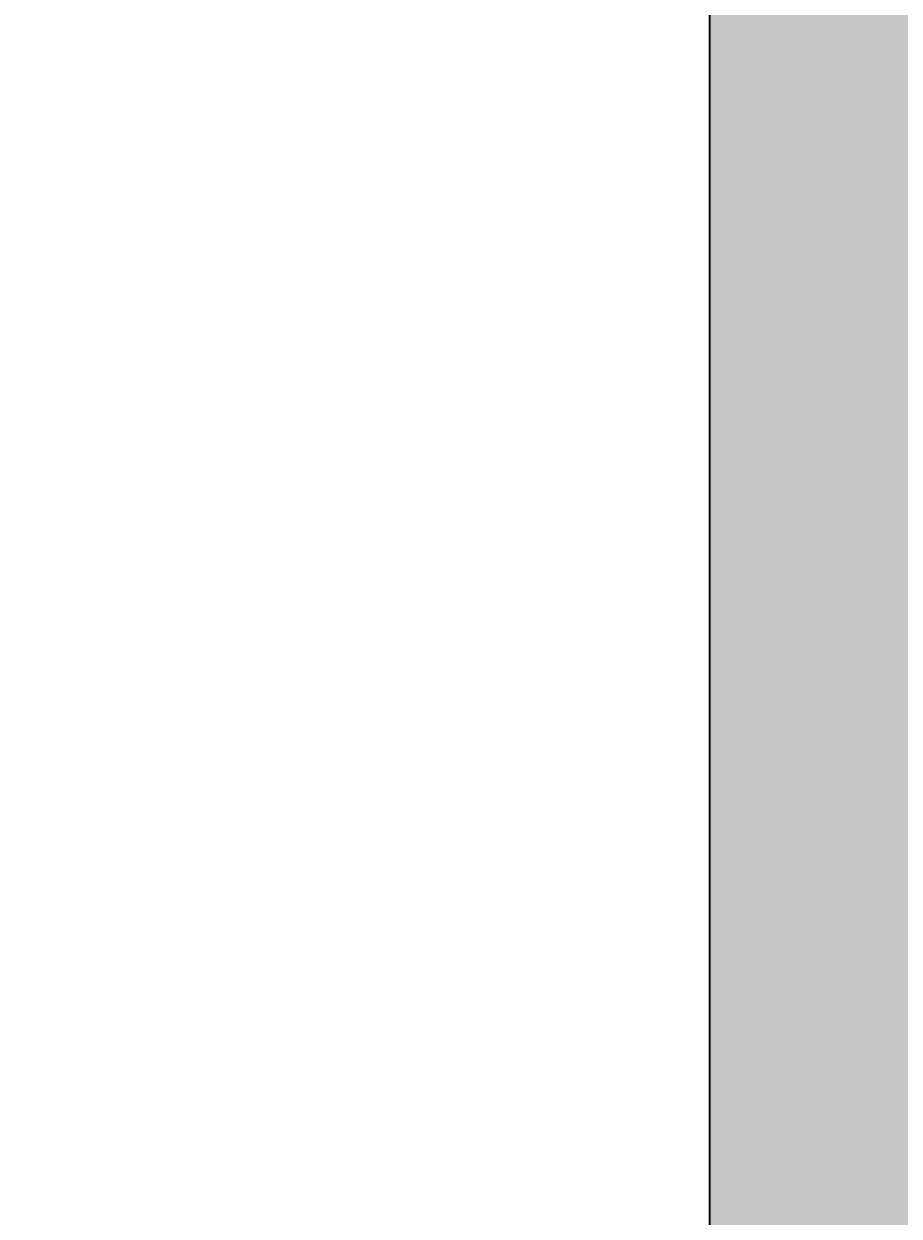
# Model space of a CAD drawing. Units: inches. Extents: x 1998 to 2588, y 1139 to 1977.
# Tile 69 of 134: x 2063 to 2095, y 1817 to 1860. Entities that reach past the tile are written whole.
import ezdxf

# ---------------------------------------------------------------- set-up
doc = ezdxf.new("R2010")
doc.units = ezdxf.units.IN
for name, color, linetype, lineweight in [('A-ANNO-DIMS', 2, 'Continuous', 18), ('A-WALL-PATT', 252, 'Continuous', 13), ('WALL', 200, 'Continuous', 35)]:
    doc.layers.add(name, color=color, linetype=linetype, lineweight=lineweight)
doc.styles.get("Standard").update_dxf_attribs({"font": 'arial.ttf'})
doc.dimstyles.get("Standard").update_dxf_attribs({"dimtxt": 0.18, "dimasz": 0.18, "dimexe": 0.18, "dimexo": 0.0625, "dimgap": 0.09, "dimtad": 0, "dimtih": 1, "dimtoh": 1, "dimdec": 4, "dimzin": 0, "dimdsep": 46, "dimtxsty": 'Standard', "dimcen": 0.09, "dimadec": 0, "dimazin": 0, "dimtfac": 1, "dimtdec": 4, "dimtofl": 0, "dimtmove": 0, "dimatfit": 3, "dimfxl": 1, "dimtolj": 1, "dimtzin": 0, "dimarcsym": 0})

# ---------------------------------------------------------------- blocks, each defined once
blk = doc.blocks.new('*D28')
at = {"layer": 'A-ANNO-DIMS', "color": 0, "lineweight": -2, "transparency": 16777216}
for p, q in [((2059.473, 1759.795), (2059.473, 1977.362)), ((2059.653, 1977.182), (2073.397, 1977.182)), ((2087.793, 1977.182), (2074.049, 1977.182)), ((2087.973, 1759.795), (2087.973, 1977.362))]:
    blk.add_line(p, q, dxfattribs=at)
at = {"layer": 'A-ANNO-DIMS', "color": 0, "transparency": 16777216}
for points in [[(2059.653, 1977.212), (2059.653, 1977.152), (2059.473, 1977.182)], [(2087.793, 1977.212), (2087.793, 1977.152), (2087.973, 1977.182)]]:
    blk.add_solid(points, dxfattribs=at)
at = {"layer": 'Defpoints', "color": 0, "transparency": 16777216}
for p in [(2087.973, 1977.182), (2059.473, 1759.732), (2087.973, 1759.732)]:
    blk.add_point(p, dxfattribs=at)
at = {"layer": 'A-ANNO-DIMS', "color": 0, "transparency": 16777216, "insert": (2073.723, 1977.182), "char_height": 0.18, "attachment_point": 5}
blk.add_mtext('\\A1;28.5', dxfattribs=at)
blk = doc.blocks.new('*D29')
at = {"layer": 'A-ANNO-DIMS', "color": 0, "lineweight": -2, "transparency": 16777216}
for p, q in [((2087.91, 1888.732), (1997.843, 1888.732)), ((1998.023, 1888.552), (1998.023, 1824.414)), ((1998.023, 1759.912), (1998.023, 1824.05)), ((2059.41, 1759.732), (1997.843, 1759.732))]:
    blk.add_line(p, q, dxfattribs=at)
at = {"layer": 'A-ANNO-DIMS', "color": 0, "transparency": 16777216}
for points in [[(1997.993, 1888.552), (1998.053, 1888.552), (1998.023, 1888.732)], [(1997.993, 1759.912), (1998.053, 1759.912), (1998.023, 1759.732)]]:
    blk.add_solid(points, dxfattribs=at)
at = {"layer": 'Defpoints', "color": 0, "transparency": 16777216}
for p in [(1998.023, 1888.732), (2087.973, 1888.732), (2059.473, 1759.732)]:
    blk.add_point(p, dxfattribs=at)
at = {"layer": 'A-ANNO-DIMS', "color": 0, "transparency": 16777216, "insert": (1998.023, 1824.232), "char_height": 0.18, "attachment_point": 5}
blk.add_mtext('\\A1;129', dxfattribs=at)

msp = doc.modelspace()

# ---------------------------------------------------------------- hatches: boundary and pattern name
at = {"layer": 'A-WALL-PATT'}
h = msp.add_hatch(color=256, dxfattribs=at)
h.dxf.hatch_style = 1
h.paths.add_polyline_path([(2222.9729, 1888.7324), (2099.4125, 1888.7324), (2099.4125, 1879.7324), (2222.9729, 1879.7324)])
h.paths.add_polyline_path([(2096.9729, 1868.3278), (2087.9729, 1868.3278), (2087.9729, 1775.637), (2096.9729, 1775.637)])
h.paths.add_polyline_path([(2227.4729, 1868.3278), (2222.9729, 1868.3278), (2222.9729, 1774.3318), (2227.4729, 1774.3318)])
h.paths.add_polyline_path([(2188.3019, 1759.7324), (2138.6074, 1759.7324), (2099.4125, 1759.7324), (2099.4125, 1755.2324), (2176.9729, 1755.2324), (2188.3019, 1755.2324)])
h.paths.add_polyline_path([(2087.9729, 1759.7324), (2059.4729, 1759.7324), (2059.4729, 1702.7324), (2087.9729, 1702.7324), (2087.9729, 1707.2324), (2063.9729, 1707.2324), (2063.9729, 1755.2324), (2087.9729, 1755.2324)])
h.paths.add_polyline_path([(2096.9729, 1755.2324), (2087.9729, 1755.2324), (2087.9729, 1707.2324), (2096.9729, 1707.2324)])
h.paths.add_polyline_path([(2187.0461, 1707.2324), (2105.9729, 1707.2324), (2096.9729, 1707.2324), (2087.9729, 1707.2324), (2087.9729, 1702.7324), (2105.9729, 1702.7324), (2114.9729, 1702.7324), (2187.0461, 1702.7324)])
h.paths.add_polyline_path([(2181.4729, 1719.2028), (2176.9729, 1719.2028), (2176.9729, 1707.2324), (2181.4729, 1707.2324)])
h.paths.add_polyline_path([(2216.0332, 1588.7324), (2114.9729, 1588.7324), (2105.9729, 1588.7324), (2105.9729, 1584.2324), (2216.0332, 1584.2324)])
h.paths.add_polyline_path([(2077.691, 1588.7324), (2061.4729, 1588.7324), (2061.4729, 1584.2324), (2077.691, 1584.2324)])
h.paths.add_polyline_path([(2105.9729, 1588.7324), (2098.0956, 1588.7324), (2098.0956, 1584.2324), (2105.9729, 1584.2324)])
h.paths.add_polyline_path([(2114.9729, 1596.2642), (2110.1012, 1596.2642), (2105.9729, 1596.2642), (2105.9729, 1588.7324), (2114.9729, 1588.7324)])
h.paths.add_polyline_path([(2114.9729, 1584.2324), (2105.9729, 1584.2324), (2105.9729, 1580.249), (2110.1012, 1580.249), (2114.9729, 1580.249)])
h.paths.add_polyline_path([(2114.9729, 1547.7716), (2110.1012, 1547.7716, -0.0318759), (2105.9729, 1548.035), (2105.9729, 1470.2324), (2108.3775, 1470.2324), (2108.3775, 1465.7324), (2186.2943, 1465.7324), (2186.2943, 1470.2324), (2114.9729, 1470.2324)])
h.paths.add_polyline_path([(2227.4729, 1584.2324), (2222.9729, 1584.2324), (2222.9729, 1486.137), (2227.4729, 1486.137)])
h.paths.add_polyline_path([(2295.4138, 1593.2324), (2227.4729, 1593.2324), (2227.4729, 1588.7324), (2295.4138, 1588.7324), (2295.4138, 1591.8729)])
h.paths.add_polyline_path([(2345.9729, 1627.1165), (2341.4729, 1627.1165), (2341.4729, 1593.2324), (2337.2869, 1593.2324), (2337.2869, 1591.8729), (2337.2869, 1588.7324), (2345.9729, 1588.7324)])
h.paths.add_polyline_path([(2291.9729, 1588.7324), (2287.4729, 1588.7324), (2287.4729, 1522.7324), (2291.9729, 1522.7324)])
h.paths.add_polyline_path([(2291.9729, 1522.7324), (2287.4729, 1522.7324), (2227.4729, 1522.7324), (2227.4729, 1518.2324), (2291.9729, 1518.2324)])
h.paths.add_polyline_path([(2295.7347, 1519.5919), (2295.7347, 1522.7324), (2291.9729, 1522.7324), (2291.9729, 1518.2324), (2295.7347, 1518.2324)])
h.paths.add_polyline_path([(2345.9729, 1522.7324), (2337.6078, 1522.7324), (2337.6078, 1519.5919), (2337.6078, 1518.2324), (2341.4729, 1518.2324), (2341.4729, 1488.5616), (2345.9729, 1488.5616)])
h.paths.add_polyline_path([(2345.9729, 1468.1569), (2341.4729, 1468.1569), (2341.4729, 1374.2324), (2227.4729, 1374.2324), (2227.4729, 1369.7324), (2345.9729, 1369.7324)])
h.paths.add_polyline_path([(2345.9729, 1369.7324), (2341.4729, 1369.7324), (2341.4729, 1362.2324), (2345.9729, 1362.2324)])
h.paths.add_polyline_path([(2345.9729, 1317.7324), (2345.9729, 1322.2324), (2341.4729, 1322.2324), (2341.4729, 1285.137), (2345.9729, 1285.137)], flags=17)
h.paths.add_polyline_path([(2356.2096, 1322.2324), (2345.9729, 1322.2324), (2345.9729, 1317.7324), (2356.2096, 1317.7324), (2356.2096, 1319.3088)], flags=17)
h.paths.add_polyline_path([(2393.9729, 1322.2324), (2375.6999, 1322.2324), (2375.6999, 1319.3088, -0.0202458), (2375.636, 1317.7324), (2393.9729, 1317.7324)], flags=17)
h.paths.add_polyline_path([(2398.4729, 1322.2324), (2393.9729, 1322.2324), (2393.9729, 1317.7324), (2393.9729, 1237.7324), (2345.9729, 1237.7324), (2345.9729, 1264.7324), (2341.4729, 1264.7324), (2341.4729, 1228.7324), (2393.9729, 1228.7324), (2482.7412, 1228.7324), (2482.7412, 1237.7324), (2398.4729, 1237.7324), (2398.4729, 1297.1029)])
h.paths.add_polyline_path([(2398.4729, 1362.2324), (2393.9729, 1362.2324), (2393.9729, 1357.7324), (2398.4729, 1357.7324)])
h.paths.add_polyline_path([(2345.9729, 1329.7549), (2341.4729, 1329.7549), (2341.4729, 1322.2324), (2345.9729, 1322.2324)])

# ---------------------------------------------------------------- linework, layer by layer
at = {"layer": 'WALL'}
msp.add_line((2087.9729, 1888.7324), (2087.9729, 1755.2324), dxfattribs=at)

# ---------------------------------------------------------------- dimensions: what is measured, and where the dimension line sits
at = {"layer": 'A-ANNO-DIMS'}
dim = msp.add_linear_dim(base=(2087.9729, 1977.1824), p1=(2059.4729, 1759.7324), p2=(2087.9729, 1759.7324), dimstyle='Standard', override={"dimdec": 1, "dimlfac": 1, "dimrnd": 0, "dimzin": 0, "dimdsep": 46, "dimlunit": 2}, dxfattribs=at)
dim.commit()
dim.dimension.update_dxf_attribs({"geometry": '*D28', "text_midpoint": (2073.7229, 1977.1824)})
dim = msp.add_linear_dim(base=(1998.0229, 1888.7324), p1=(2059.4729, 1759.7324), p2=(2087.9729, 1888.7324), angle=90, dimstyle='Standard', override={"dimdec": 0, "dimlfac": 1, "dimrnd": 0, "dimzin": 0, "dimdsep": 46, "dimlunit": 2}, dxfattribs=at)
dim.commit()
dim.dimension.update_dxf_attribs({"geometry": '*D29', "text_midpoint": (1998.0229, 1824.2324)})

doc.saveas('drawing.dxf')
